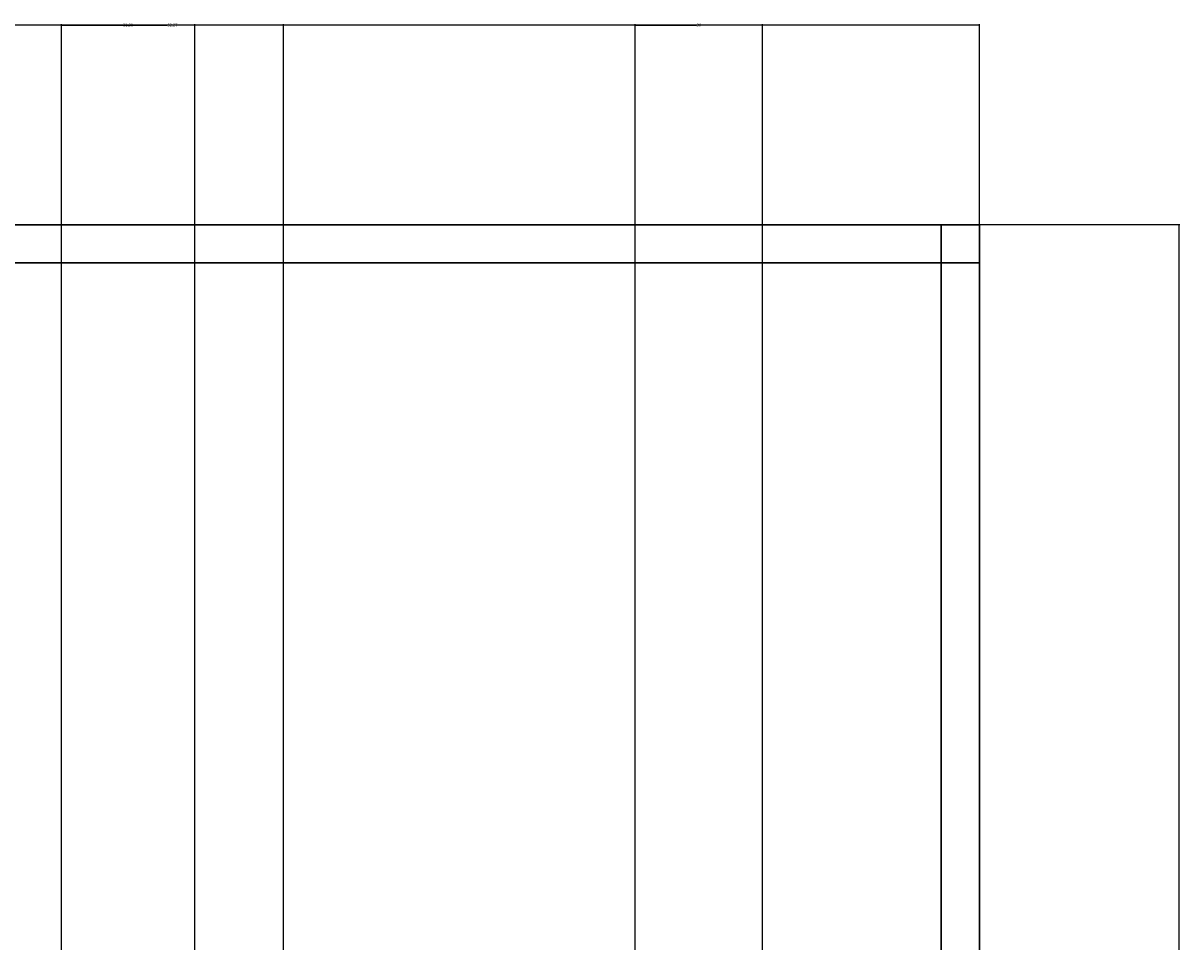
# Model space of a CAD drawing. Units: inches. Extents: x 867 to 1667, y -234 to 788.
# Tile 42 of 42: x 1395 to 1667, y 572 to 788. Entities that reach past the tile are written whole.
import ezdxf

# ---------------------------------------------------------------- set-up
doc = ezdxf.new("R2010")
doc.units = ezdxf.units.IN
doc.header["$MEASUREMENT"] = 0
doc.layers.add('A-ANNO-DIMS', color=2, linetype='Continuous', lineweight=18)
doc.layers.add('A-WALL-SITE', color=8, linetype='Continuous', lineweight=30)
doc.styles.get("Standard").update_dxf_attribs({"font": 'arial.ttf'})
doc.dimstyles.get("Standard").update_dxf_attribs({"dimtxt": 0.6875, "dimasz": 0.18, "dimexe": 0.18, "dimexo": 0.0625, "dimgap": 0.09, "dimtad": 0, "dimdec": 4, "dimzin": 0, "dimdsep": 46, "dimlunit": 4, "dimtxsty": 'Standard', "dimcen": 0.09, "dimadec": 0, "dimazin": 0, "dimtfac": 1, "dimtdec": 4, "dimtofl": 0, "dimtmove": 0, "dimatfit": 3, "dimfxl": 1, "dimtolj": 1, "dimtzin": 0, "dimarcsym": 0})

# ---------------------------------------------------------------- blocks, each defined once
blk = doc.blocks.new('*D17')
at = {"layer": 'A-ANNO-DIMS', "color": 0, "lineweight": -2, "transparency": 16777216}
for p, q in [((914.89, 740.68), (914.89, 787.75)), ((915.07, 787.57), (1266.54, 787.57)), ((1619.71, 787.57), (1268.24, 787.57)), ((1619.89, 740.68), (1619.89, 787.75))]:
    blk.add_line(p, q, dxfattribs=at)
at = {"layer": 'A-ANNO-DIMS', "color": 0, "transparency": 16777216}
for points in [[(915.07, 787.6), (915.07, 787.54), (914.89, 787.57)], [(1619.71, 787.6), (1619.71, 787.54), (1619.89, 787.57)]]:
    blk.add_solid(points, dxfattribs=at)
at = {"layer": 'Defpoints', "color": 0, "transparency": 16777216}
for p in [(1619.89, 787.57), (914.89, 740.62), (1619.89, 740.62)]:
    blk.add_point(p, dxfattribs=at)
at = {"layer": 'A-ANNO-DIMS', "color": 0, "transparency": 16777216, "insert": (1267.39, 787.57), "char_height": 0.688, "attachment_point": 5}
blk.add_mtext('\\A1;705', dxfattribs=at)
blk = doc.blocks.new('*D18')
at = {"layer": 'A-ANNO-DIMS', "color": 0, "lineweight": -2, "transparency": 16777216}
for p, q in [((1619.95, 740.62), (1667.02, 740.62)), ((1666.84, 740.44), (1666.84, 277.95)), ((1666.84, -186.23), (1666.84, 276.25)), ((1619.95, -186.41), (1667.02, -186.41))]:
    blk.add_line(p, q, dxfattribs=at)
at = {"layer": 'A-ANNO-DIMS', "color": 0, "transparency": 16777216}
for points in [[(1666.81, 740.44), (1666.87, 740.44), (1666.84, 740.62)], [(1666.81, -186.23), (1666.87, -186.23), (1666.84, -186.41)]]:
    blk.add_solid(points, dxfattribs=at)
at = {"layer": 'Defpoints', "color": 0, "transparency": 16777216}
for p in [(1619.89, 740.62), (1666.84, 740.62), (1619.89, -186.41)]:
    blk.add_point(p, dxfattribs=at)
at = {"layer": 'A-ANNO-DIMS', "color": 0, "transparency": 16777216, "insert": (1666.84, 277.1), "char_height": 0.688, "attachment_point": 5, "rotation": 90}
blk.add_mtext('\\A1;927', dxfattribs=at)
blk = doc.blocks.new('*D31')
at = {"layer": 'A-ANNO-DIMS', "color": 0, "lineweight": -2, "transparency": 16777216}
for p, q in [((1070.89, 566.68), (1070.89, 787.75)), ((1071.07, 787.57), (1304.02, 787.57)), ((1538.71, 787.57), (1305.75, 787.57)), ((1538.89, 566.68), (1538.89, 787.75))]:
    blk.add_line(p, q, dxfattribs=at)
at = {"layer": 'A-ANNO-DIMS', "color": 0, "transparency": 16777216}
for points in [[(1071.07, 787.6), (1071.07, 787.54), (1070.89, 787.57)], [(1538.71, 787.6), (1538.71, 787.54), (1538.89, 787.57)]]:
    blk.add_solid(points, dxfattribs=at)
at = {"layer": 'Defpoints', "color": 0, "transparency": 16777216}
for p in [(1538.89, 787.57), (1070.89, 566.62), (1538.89, 566.62)]:
    blk.add_point(p, dxfattribs=at)
at = {"layer": 'A-ANNO-DIMS', "color": 0, "transparency": 16777216, "insert": (1304.89, 787.57), "char_height": 0.688, "attachment_point": 5}
blk.add_mtext('\\A1;468', dxfattribs=at)
blk = doc.blocks.new('*D36')
at = {"layer": 'A-ANNO-DIMS', "color": 0, "lineweight": -2, "transparency": 16777216}
for p, q in [((1538.89, 413.68), (1538.89, 787.75)), ((1539.07, 787.57), (1553.31, 787.57)), ((1568.71, 787.57), (1554.47, 787.57)), ((1568.89, 413.68), (1568.89, 787.75))]:
    blk.add_line(p, q, dxfattribs=at)
at = {"layer": 'A-ANNO-DIMS', "color": 0, "transparency": 16777216}
for points in [[(1539.07, 787.6), (1539.07, 787.54), (1538.89, 787.57)], [(1568.71, 787.6), (1568.71, 787.54), (1568.89, 787.57)]]:
    blk.add_solid(points, dxfattribs=at)
at = {"layer": 'Defpoints', "color": 0, "transparency": 16777216}
for p in [(1568.89, 787.57), (1538.89, 413.62), (1568.89, 413.62)]:
    blk.add_point(p, dxfattribs=at)
at = {"layer": 'A-ANNO-DIMS', "color": 0, "transparency": 16777216, "insert": (1553.89, 787.57), "char_height": 0.688, "attachment_point": 5}
blk.add_mtext('\\A1;30', dxfattribs=at)
blk = doc.blocks.new('*D53')
at = {"layer": 'A-ANNO-DIMS', "color": 0, "lineweight": -2, "transparency": 16777216}
for p, q in [((1403.89, 557.68), (1403.89, 787.75)), ((1404.07, 787.57), (1418.33, 787.57)), ((1435.1, 787.57), (1420.83, 787.57)), ((1435.28, 557.68), (1435.28, 787.75))]:
    blk.add_line(p, q, dxfattribs=at)
at = {"layer": 'A-ANNO-DIMS', "color": 0, "transparency": 16777216}
for points in [[(1404.07, 787.6), (1404.07, 787.54), (1403.89, 787.57)], [(1435.1, 787.6), (1435.1, 787.54), (1435.28, 787.57)]]:
    blk.add_solid(points, dxfattribs=at)
at = {"layer": 'Defpoints', "color": 0, "transparency": 16777216}
for p in [(1403.89, 787.57), (1403.89, 557.62), (1435.28, 557.62)]:
    blk.add_point(p, dxfattribs=at)
at = {"layer": 'A-ANNO-DIMS', "color": 0, "transparency": 16777216, "insert": (1419.58, 787.57), "char_height": 0.688, "attachment_point": 5}
blk.add_mtext('\\A1;31.39', dxfattribs=at)
blk = doc.blocks.new('*D54')
at = {"layer": 'A-ANNO-DIMS', "color": 0, "lineweight": -2, "transparency": 16777216}
for p, q in [((1403.89, 413.68), (1403.89, 787.75)), ((1404.07, 787.57), (1428.77, 787.57)), ((1455.97, 787.57), (1431.27, 787.57)), ((1456.15, 413.68), (1456.15, 787.75))]:
    blk.add_line(p, q, dxfattribs=at)
at = {"layer": 'A-ANNO-DIMS', "color": 0, "transparency": 16777216}
for points in [[(1404.07, 787.6), (1404.07, 787.54), (1403.89, 787.57)], [(1455.97, 787.6), (1455.97, 787.54), (1456.15, 787.57)]]:
    blk.add_solid(points, dxfattribs=at)
at = {"layer": 'Defpoints', "color": 0, "transparency": 16777216}
for p in [(1456.15, 787.57), (1403.89, 413.62), (1456.15, 413.62)]:
    blk.add_point(p, dxfattribs=at)
at = {"layer": 'A-ANNO-DIMS', "color": 0, "transparency": 16777216, "insert": (1430.02, 787.57), "char_height": 0.688, "attachment_point": 5}
blk.add_mtext('\\A1;52.27', dxfattribs=at)

msp = doc.modelspace()

# ---------------------------------------------------------------- linework, layer by layer
at = {"layer": 'A-WALL-SITE'}
for p, q in [((1619.8866, 740.617), (914.8866, 740.617)), ((1610.8866, 740.617), (1610.8866, -186.4081)), ((1619.8866, 740.617), (1619.8866, -186.4081)), ((1619.8866, 731.617), (914.8866, 731.617))]:
    msp.add_line(p, q, dxfattribs=at)

# ---------------------------------------------------------------- dimensions: what is measured, and where the dimension line sits
at = {"layer": 'A-ANNO-DIMS'}
for base, p1, p2, override, picture, middle in [((1619.8866, 787.567), (914.8866, 740.617), (1619.8866, 740.617), {"dimdec": 0, "dimlfac": 1, "dimrnd": 0, "dimzin": 0, "dimdsep": 46, "dimlunit": 2}, '*D17', (1267.3866, 787.567)), ((1538.8866, 787.567), (1070.8866, 566.617), (1538.8866, 566.617), {"dimdec": 0, "dimlfac": 1, "dimrnd": 0, "dimzin": 0, "dimdsep": 46, "dimlunit": 2}, '*D31', (1304.8866, 787.567)), ((1403.8866, 787.567), (1435.2754, 557.617), (1403.8866, 557.617), {"dimdec": 2, "dimlfac": 1, "dimrnd": 0, "dimzin": 0, "dimdsep": 46, "dimlunit": 2}, '*D53', (1419.581, 787.567)), ((1456.1541, 787.567), (1403.8866, 413.617), (1456.1541, 413.617), {"dimdec": 2, "dimlfac": 1, "dimrnd": 0, "dimzin": 0, "dimdsep": 46, "dimlunit": 2}, '*D54', (1430.0204, 787.567)), ((1568.8866, 787.567), (1538.8866, 413.617), (1568.8866, 413.617), {"dimdec": 0, "dimlfac": 1, "dimrnd": 0, "dimzin": 0, "dimdsep": 46, "dimlunit": 2}, '*D36', (1553.8866, 787.567))]:
    dim = msp.add_linear_dim(base=base, p1=p1, p2=p2, dimstyle='Standard', override=override, dxfattribs=at)
    dim.commit()
    dim.dimension.update_dxf_attribs({"geometry": picture, "text_midpoint": middle})
dim = msp.add_linear_dim(base=(1666.8366, 740.617), p1=(1619.8866, -186.4081), p2=(1619.8866, 740.617), angle=90, dimstyle='Standard', override={"dimdec": 0, "dimlfac": 1, "dimrnd": 0, "dimzin": 0, "dimdsep": 46, "dimlunit": 2}, dxfattribs=at)
dim.commit()
dim.dimension.update_dxf_attribs({"geometry": '*D18', "text_midpoint": (1666.8366, 277.1045)})

doc.saveas('drawing.dxf')
